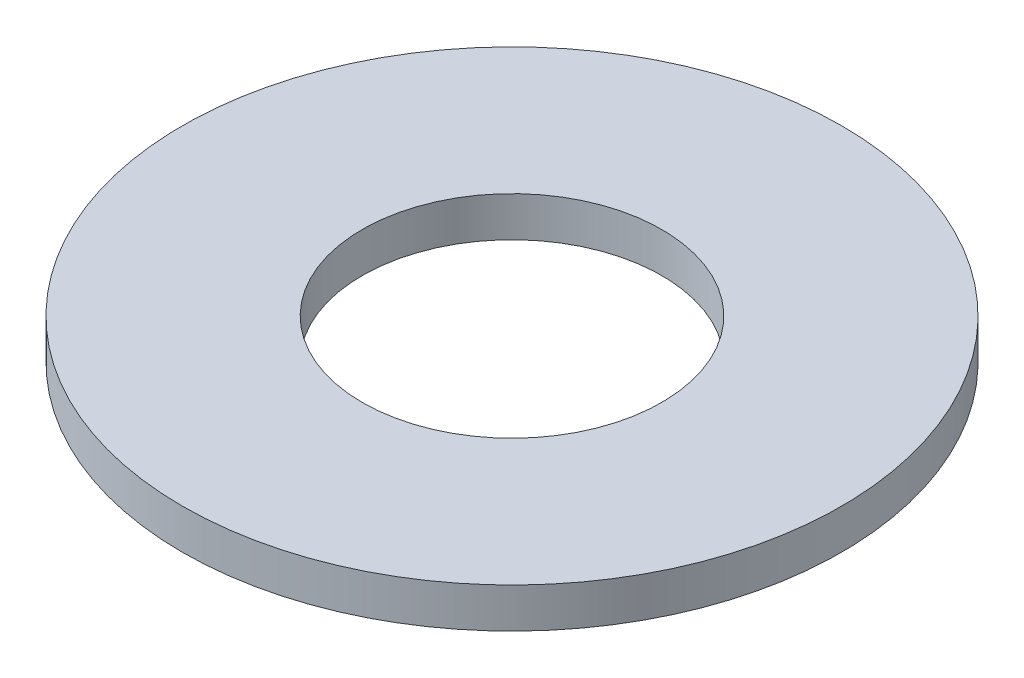
SolidWorks part; units mm, degrees
material "Galvanized Steel"
ref_plane "Front Plane" through (0, 0, 0) normal (0, 0, 1) x (1, 0, 0)
ref_plane "Top Plane" through (0, 0, 0) normal (0, 1, 0) x (1, 0, 0)
ref_plane "Right Plane" through (0, 0, 0) normal (1, 0, 0) x (0, 0, -1)
sketch "Washer Profile Ø165xØ75" plane through (0, 0, 0) normal (0, 1, 0) x (1, 0, 0)
  circle A0 centre (0, 0) radius 82.5
  circle A1 centre (0, 0) radius 37.5
  dimension "D1" = 165
  dimension "D2" = 75
extrude "Washer Body 10mm" add sketch "Washer Profile Ø165xØ75" along normal blind 10
